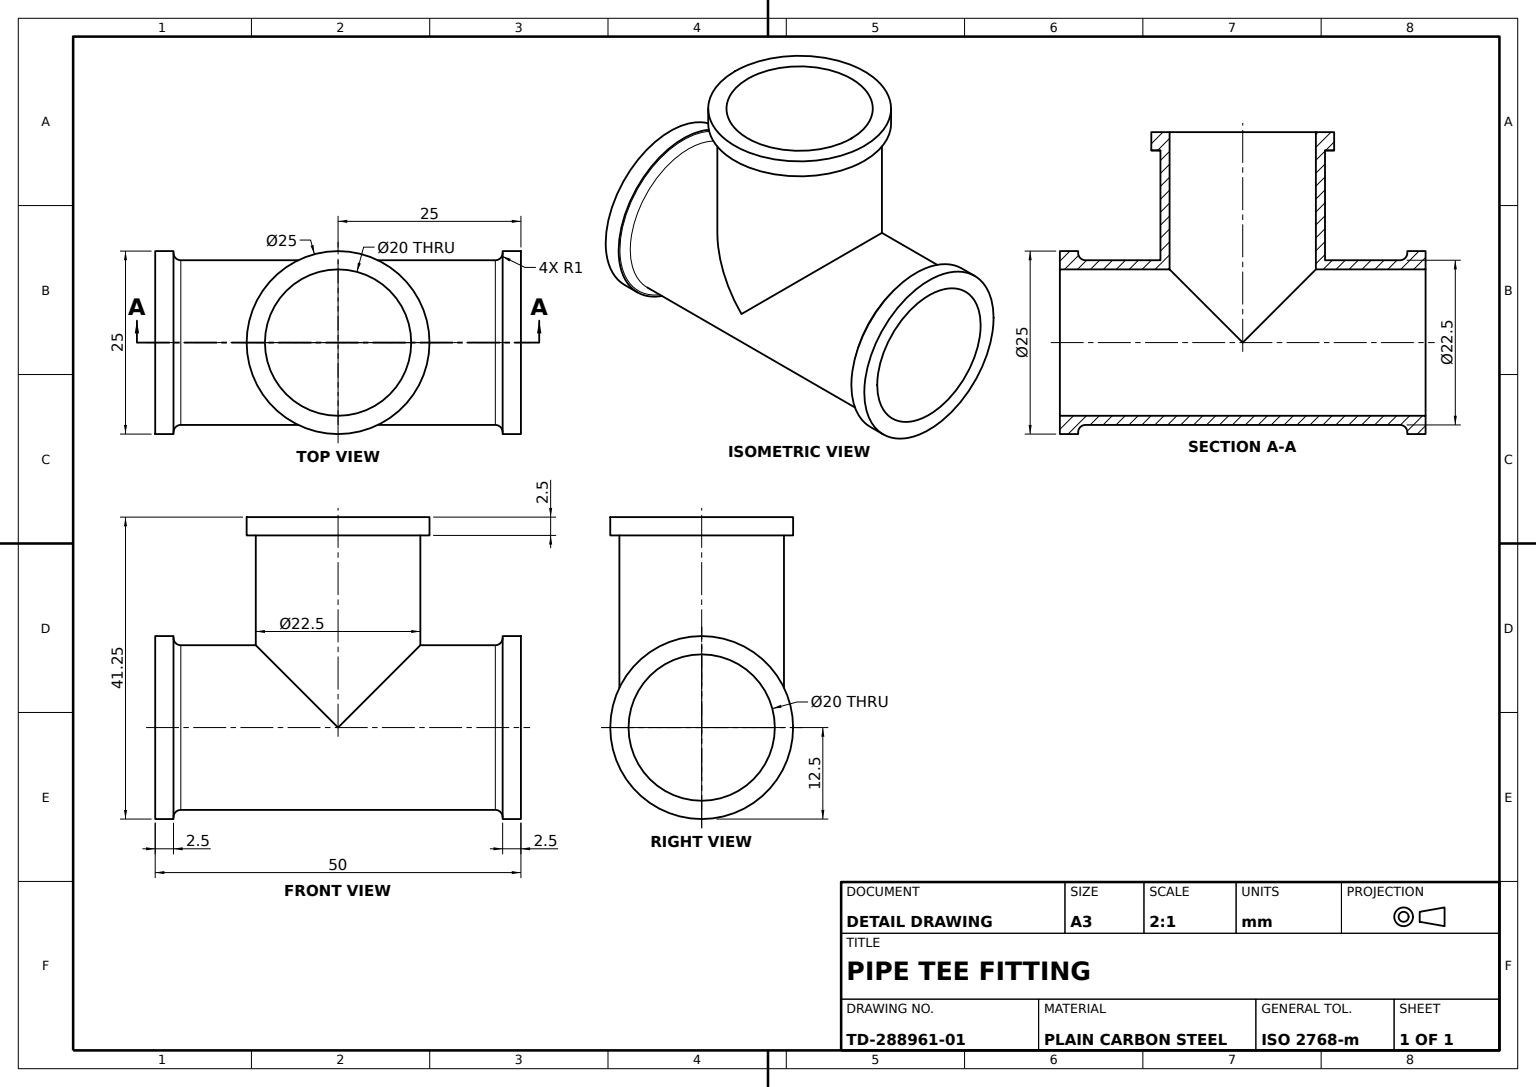
from build123d import *

# Parameters (mm, degrees)
END_RIM_A_PROFILE_25_R       = 12.5
END_RIM_A_25_DEPTH           = 1.25
RUN_START                    = -2.5
RUN_TUBE_PROFILE_22_5_R      = 11.25
RUN_TUBE_22_5_DEPTH          = 45
END_RIM_B_PROFILE_25_R       = 12.5
END_RIM_B_25_DEPTH           = 2.5
RUN_BORE_PROFILE_20_R        = 10
RUN_BORE_20_DEPTH            = 54.033008589
RIM_FILLETS_R1_R             = 1
BRANCH_START                 = 26.25
BRANCH_RIM_25_DEPTH          = 2.5
BRANCH_TUBE_PROFILE_22_5_R   = 11.25
BRANCH_TUBE_22_5_DEPTH       = 27
RUN_BORE_CLEARANCE_PROFILE_R = 10
RUN_BORE_CLEARANCE_CUT_DEPTH = 60.015358255
BRANCH_BORE_20_REACH         = 67.072
BRANCH_BORE_20_END_RADIUS    = 10
BRANCH_BORE_PROFILE_20_R     = 10


with BuildPart() as part:
    # End Rim A Profile Ø25 → End Rim A Ø25 (new, symmetric)
    with BuildSketch(Plane.XY):
        Circle(END_RIM_A_PROFILE_25_R)
    extrude(amount=END_RIM_A_25_DEPTH, both=True)

    # Run Tube Profile Ø22.5 → Run Tube Ø22.5 (add)
    with BuildSketch(Plane.XY.offset(1.25).offset(RUN_START)):
        Circle(RUN_TUBE_PROFILE_22_5_R)
    extrude(amount=-RUN_TUBE_22_5_DEPTH)

    # End Rim B Profile Ø25 → End Rim B Ø25 (add)
    with BuildSketch(Plane(origin=(0, 0, -46.25), x_dir=(-1, 0, 0), z_dir=(0, 0, -1))):
        with Locations(Location((0, 0, 0), (0, 0, 180))):
            Circle(END_RIM_B_PROFILE_25_R)
    extrude(amount=END_RIM_B_25_DEPTH)

    # Run Bore Profile Ø20 → Run Bore Ø20 (cut, through all)
    with BuildSketch(Plane(origin=(0, 0, -48.75), x_dir=(-1, 0, 0), z_dir=(0, 0, -1))):
        Circle(RUN_BORE_PROFILE_20_R)
    extrude(amount=-RUN_BORE_20_DEPTH, mode=Mode.SUBTRACT)

    # Rim Fillets R1
    rim_fillets_r1_edges = [part.edges().sort_by_distance(p)[0] for p in [
        (-11.25, 0, -46.25),
        (-11.25, 0, -1.25),
    ]]
    fillet(rim_fillets_r1_edges, radius=RIM_FILLETS_R1_R)



with BuildPart() as body_2:
    # Branch Rim Profile Ø25 → Branch Rim Ø25 (new body)
    with BuildSketch(Plane(origin=(0, 0, 0), x_dir=(1, 0, 0), z_dir=(0, 1, 0)).offset(BRANCH_START)):
        with BuildLine():
            ThreePointArc((12.5, 23.75), (8.838834765, 32.588834765), (0, 36.25))
            Line((0, 36.25), (0, 11.25))
            ThreePointArc((0, 11.25), (8.838834765, 14.911165235), (12.5, 23.75))
        make_face()
        with BuildLine():
            Line((0, 11.25), (0, 36.25))
            ThreePointArc((0, 36.25), (-12.5, 23.75), (0, 11.25))
        make_face()
    extrude(amount=BRANCH_RIM_25_DEPTH)


with BuildPart() as part_1:
    add(part.part)

    add(body_2.part)  # Branch Tube Ø22.5 merges body 2
    # Branch Tube Profile Ø22.5 → Branch Tube Ø22.5 (add)
    with BuildSketch(Plane(origin=(0, 0, 0), x_dir=(1, 0, 0), z_dir=(0, 1, 0))):
        with Locations((0, 23.75)):
            Circle(BRANCH_TUBE_PROFILE_22_5_R)
    extrude(amount=BRANCH_TUBE_22_5_DEPTH)

    # Run Bore Clearance Profile → Run Bore Clearance Cut (cut, through all)
    with BuildSketch(Plane.XY.offset(1.25)):
        with Locations(Location((0, 0, 0), (0, 0, 180))):
            Circle(RUN_BORE_CLEARANCE_PROFILE_R)
    extrude(amount=-RUN_BORE_CLEARANCE_CUT_DEPTH, mode=Mode.SUBTRACT)

    # Branch Bore Ø20: up to this cylinder (the profile starts outside it)
    branch_bore_20_end = Plane(origin=(0, 0, -23.75), z_dir=(0, 0, -1)) * Cylinder(BRANCH_BORE_20_END_RADIUS, 155.144, mode=Mode.PRIVATE)
    # Branch Bore Profile Ø20 → Branch Bore Ø20 (cut, up to the surface)
    with BuildSketch(Plane(origin=(0, 28.75, 0), x_dir=(1, 0, 0), z_dir=(0, 1, 0)), mode=Mode.PRIVATE) as branch_bore_20_sk1:
        with Locations(Location((0, 23.75, 0), (0, 0, 270))):
            Circle(BRANCH_BORE_PROFILE_20_R)
    branch_bore_20_tool1 = extrude(branch_bore_20_sk1.sketch, amount=-BRANCH_BORE_20_REACH, mode=Mode.PRIVATE) - branch_bore_20_end
    add(branch_bore_20_tool1.solids().sort_by_distance((0, 28.75, -23.75))[0], mode=Mode.SUBTRACT)


solid = part_1.part
